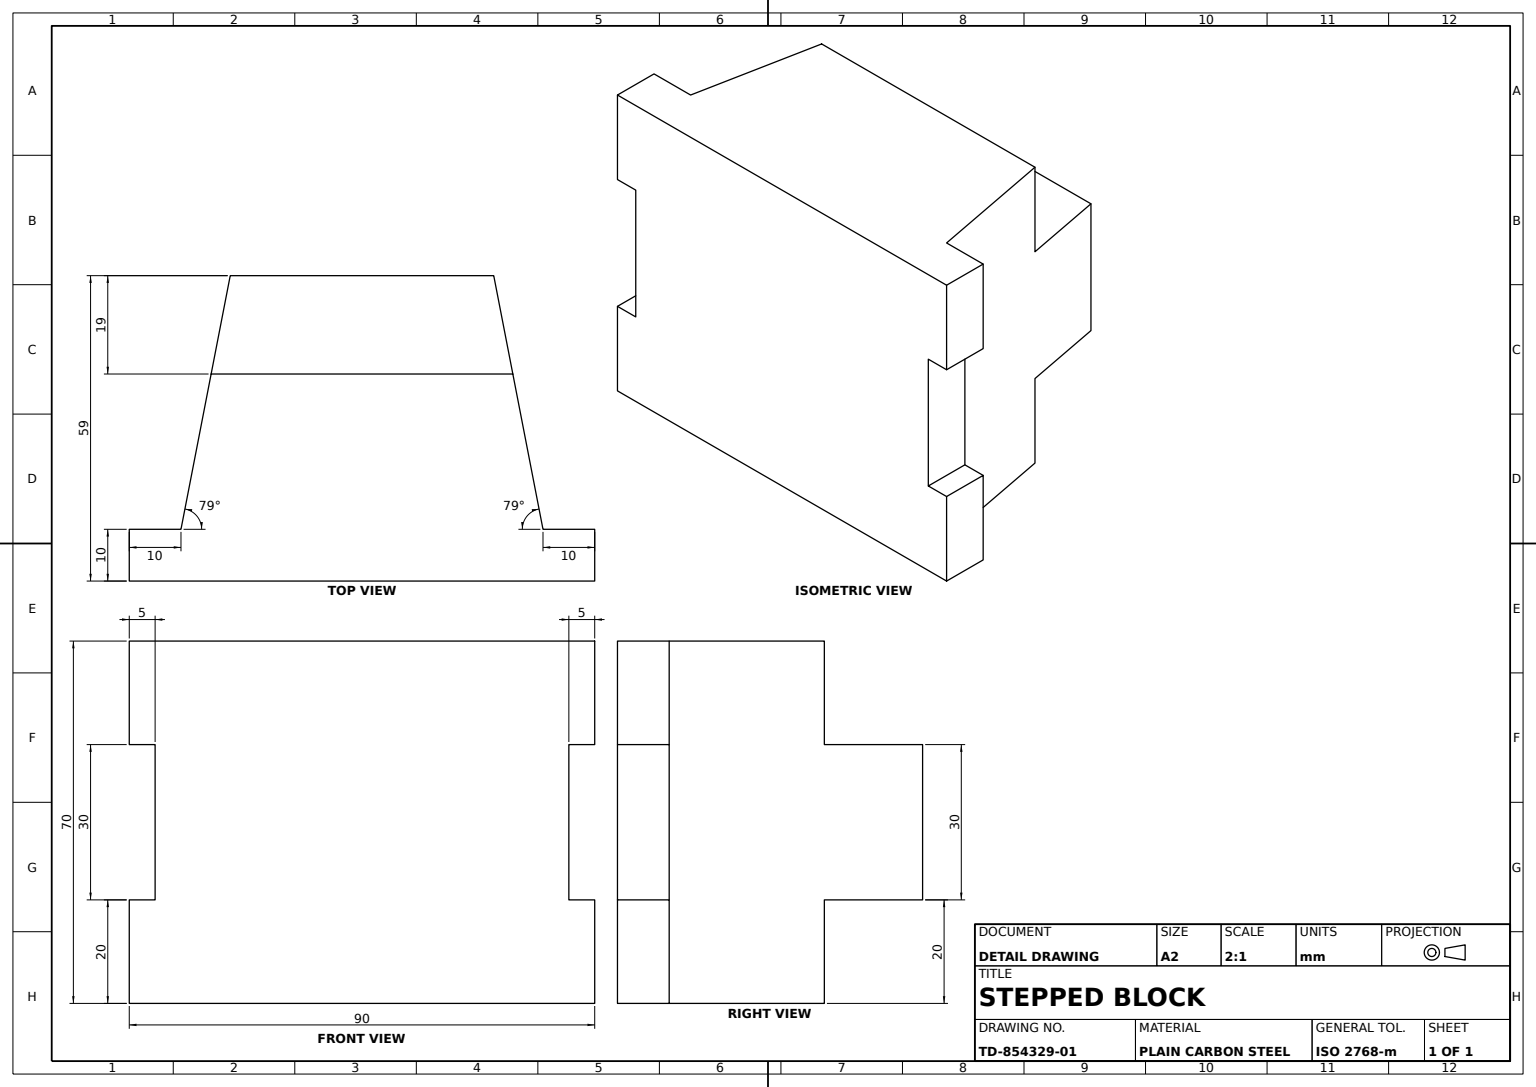
from build123d import *

# Parameters (mm, degrees)
BASE_PLATE_DEPTH        = 10
TAPERED_BOSS_DEPTH      = 70
TOP_SLOT_PROFILE_W      = 92.427210419
TOP_SLOT_PROFILE_H      = 20
TOP_SLOT_PROFILE_W_2    = 89.987361697
TOP_SLOT_CUT_19MM_DEPTH = 19


with BuildPart() as part:
    # Base Plate Profile → Base Plate (new body)
    with BuildSketch(Plane.XY):
        Polygon((-45, -15), (-45, -35), (45, -35), (45, -15), (40, -15), (40, 15), (45, 15), (45, 35), (-45, 35), (-45, 15), (-40, 15), (-40, -15), align=None)
    extrude(amount=BASE_PLATE_DEPTH)

    # Tapered Boss Profile → Tapered Boss (add)
    with BuildSketch(Plane(origin=(0, 35, 0), x_dir=(1, 0, 0), z_dir=(0, 1, 0))):
        Polygon((-25.475364852, 49), (-35, 0), (35, 0), (25.475364852, 49), align=None)
    extrude(amount=-TAPERED_BOSS_DEPTH)

    # Top Slot Profile → Top Slot Cut 19mm (cut)
    with BuildSketch(Plane(origin=(0, 0, -49), x_dir=(-1, 0, 0), z_dir=(0, 0, -1))):
        with Locations((7.299783504, 25)):
            Rectangle(TOP_SLOT_PROFILE_W, TOP_SLOT_PROFILE_H)
        with Locations((6.079859143, -25)):
            Rectangle(TOP_SLOT_PROFILE_W_2, TOP_SLOT_PROFILE_H)
    extrude(amount=-TOP_SLOT_CUT_19MM_DEPTH, mode=Mode.SUBTRACT)


solid = part.part
